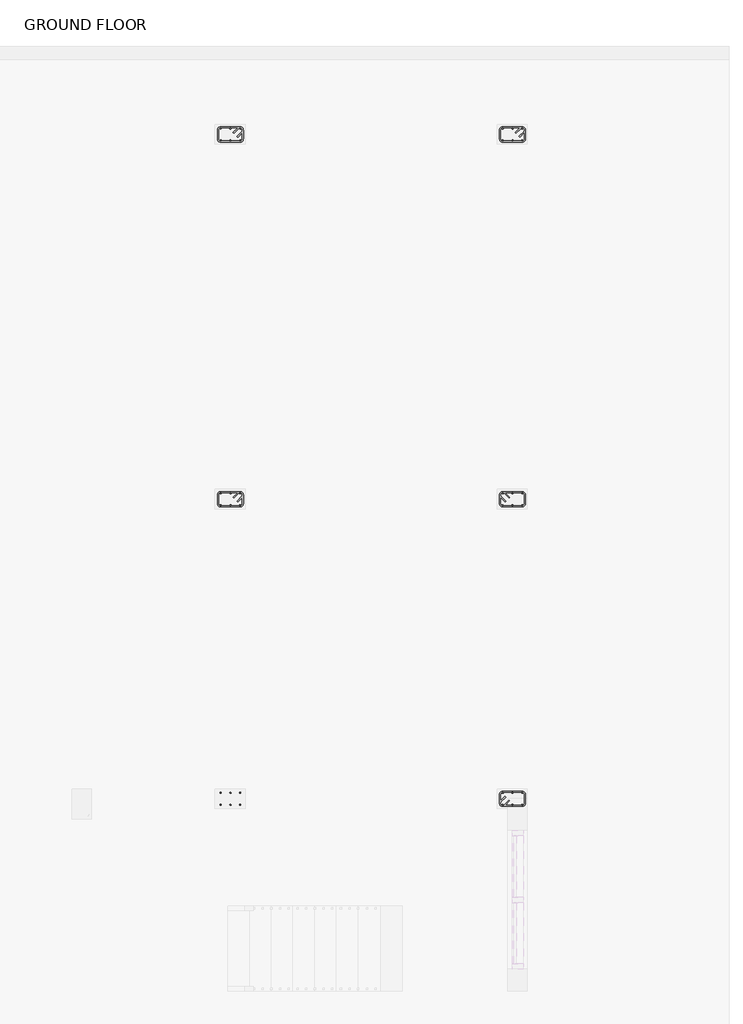
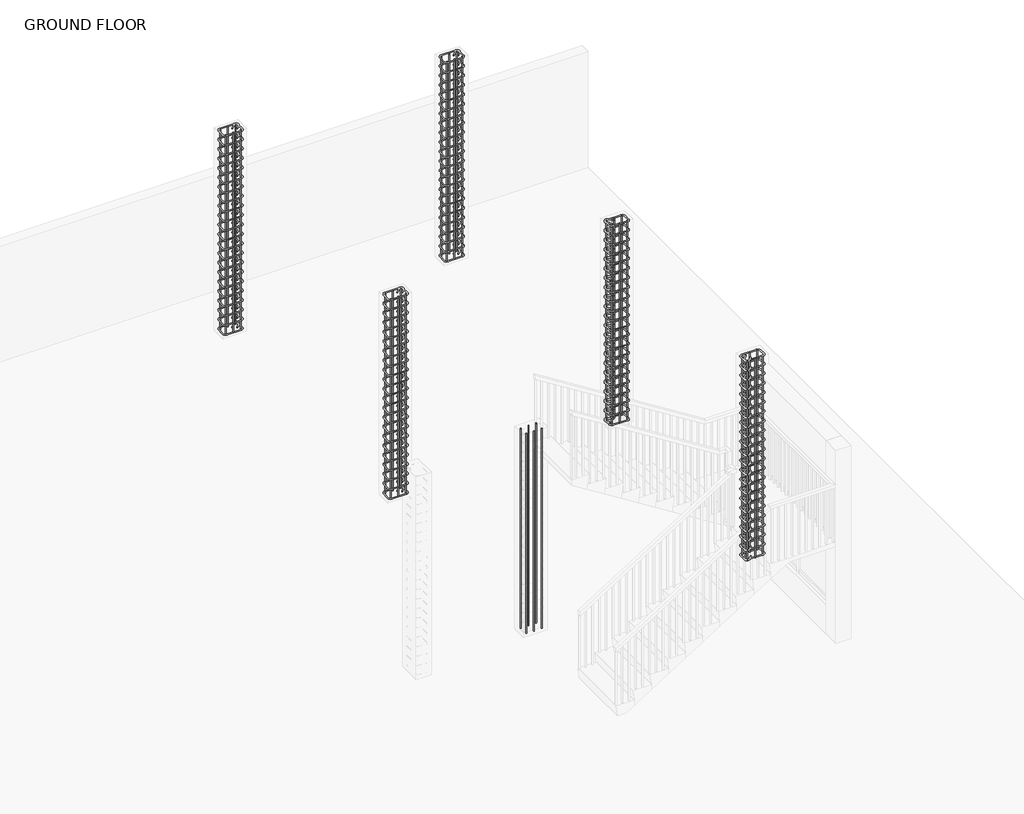
# One storey, part 7 of 7: 17 reinforcing bars.
"""IFC4 building model written with IfcOpenShell, lengths in millimetres."""

from ifc_helpers import new_model, si_unit, point, frame, origin, place, context, project, spatial, polyline, circle_curve, trimmed, segment, composite_curve, source, transform, mapped, element, save
from ifc_brep_helpers import swept_disk

model = new_model("IFC4")

# Units and contexts
model_context = context("Model", 3, world=origin())
ifc_project = project(units=[si_unit("LENGTHUNIT", "METRE", prefix="MILLI")], contexts=[model_context])

# Site, building, storey
site = spatial("IfcSite", under=ifc_project)
building = spatial("IfcBuilding", under=site)
storey = spatial("IfcBuildingStorey", under=building, Name="GROUND FLOOR", Elevation=0.0)

# Reinforcing bars
placement = place(None, origin())
reinforcing_bar_shape = source(origin(), model_context, "Body", "SolidModel", [
    swept_disk(composite_curve([segment(polyline([(4498.0475177, 5737.027757, 3168.65), (4444.165981, 5790.9092937, 3168.65)]), True, "CONTINUOUS"), segment(trimmed(circle_curve(frame((4466.6166213, 5813.359934, 3168.65), z_axis=(0.0, 0.0, -1.0), x_axis=(-22.450640299999577, -22.450640300000487, 0.0)), 31.75), [point((4444.165981, 5790.9092937, 3168.65))], [point((4466.6166213, 5845.109934, 3168.65))], True, "CARTESIAN"), True, "CONTINUOUS"), segment(polyline([(4466.6166213, 5845.109934, 3168.65), (4695.2166213, 5845.109934, 3168.65)]), True, "CONTINUOUS"), segment(trimmed(circle_curve(frame((4695.2166213, 5813.359934, 3168.65), z_axis=(0.0, 0.0, -1.0), x_axis=(0.0, 31.75, 0.0)), 31.75), [point((4695.2166213, 5845.109934, 3168.65))], [point((4726.9666213, 5813.359934, 3168.65))], True, "CARTESIAN"), True, "CONTINUOUS"), segment(polyline([(4726.9666213, 5813.359934, 3168.65), (4726.9666213, 5711.759934, 3168.65)]), True, "CONTINUOUS"), segment(trimmed(circle_curve(frame((4695.2465882, 5711.759934, 3170.0291319), z_axis=(-0.043437224276306856, 0.0, -0.9990561583550596), x_axis=(31.720033100000364, 0.0, -1.3791318999997202)), 31.75), [point((4726.9666213, 5711.759934, 3168.65))], [point((4695.2465882, 5680.009934, 3170.0291319))], True, "CARTESIAN"), True, "CONTINUOUS"), segment(polyline([(4695.2465882, 5680.009934, 3170.0291319), (4466.5866543, 5680.009934, 3179.9708681)]), True, "CONTINUOUS"), segment(trimmed(circle_curve(frame((4466.5866543, 5711.759934, 3179.9708681), z_axis=(-0.043437224276306856, 0.0, -0.9990561583550596), x_axis=(0.0, -31.75, 0.0)), 31.75), [point((4466.5866543, 5680.009934, 3179.9708681))], [point((4434.8666213, 5711.759934, 3181.35))], True, "CARTESIAN"), True, "CONTINUOUS"), segment(polyline([(4434.8666213, 5711.759934, 3181.35), (4434.8666213, 5813.359934, 3181.35)]), True, "CONTINUOUS"), segment(trimmed(circle_curve(frame((4466.6166213, 5813.359934, 3181.35), z_axis=(0.0, 0.0, -1.0), x_axis=(-31.75, 0.0, 0.0)), 31.75), [point((4434.8666213, 5813.359934, 3181.35))], [point((4489.0672616, 5835.8105743, 3181.35))], True, "CARTESIAN"), True, "CONTINUOUS"), segment(polyline([(4489.0672616, 5835.8105743, 3181.35), (4542.9487983, 5781.9290376, 3181.35)]), True, "CONTINUOUS")], self_intersect=False), 6.35),
])
element("IfcReinforcingBar", 1, at=placement, inside=storey, context=model_context, shape_type="MappedRepresentation", body=[
    mapped(reinforcing_bar_shape, transform((0.0, 0.0, 0.0), x_axis=(1.0, 0.0, 0.0), y_axis=(0.0, 1.0, 0.0), z_axis=(0.0, 0.0, 1.0))),
    mapped(reinforcing_bar_shape, transform((0.0, 0.0, -149.3761905), x_axis=(1.0, 0.0, 0.0), y_axis=(0.0, 1.0, 0.0), z_axis=(0.0, 0.0, 1.0))),
    mapped(reinforcing_bar_shape, transform((0.0, 0.0, -298.752381), x_axis=(1.0, 0.0, 0.0), y_axis=(0.0, 1.0, 0.0), z_axis=(0.0, 0.0, 1.0))),
    mapped(reinforcing_bar_shape, transform((0.0, 0.0, -448.1285714), x_axis=(1.0, 0.0, 0.0), y_axis=(0.0, 1.0, 0.0), z_axis=(0.0, 0.0, 1.0))),
    mapped(reinforcing_bar_shape, transform((0.0, 0.0, -597.5047619), x_axis=(1.0, 0.0, 0.0), y_axis=(0.0, 1.0, 0.0), z_axis=(0.0, 0.0, 1.0))),
    mapped(reinforcing_bar_shape, transform((0.0, 0.0, -746.8809524), x_axis=(1.0, 0.0, 0.0), y_axis=(0.0, 1.0, 0.0), z_axis=(0.0, 0.0, 1.0))),
    mapped(reinforcing_bar_shape, transform((0.0, 0.0, -896.2571429), x_axis=(1.0, 0.0, 0.0), y_axis=(0.0, 1.0, 0.0), z_axis=(0.0, 0.0, 1.0))),
    mapped(reinforcing_bar_shape, transform((0.0, 0.0, -1045.6333333), x_axis=(1.0, 0.0, 0.0), y_axis=(0.0, 1.0, 0.0), z_axis=(0.0, 0.0, 1.0))),
    mapped(reinforcing_bar_shape, transform((0.0, 0.0, -1195.0095238), x_axis=(1.0, 0.0, 0.0), y_axis=(0.0, 1.0, 0.0), z_axis=(0.0, 0.0, 1.0))),
    mapped(reinforcing_bar_shape, transform((0.0, 0.0, -1344.3857143), x_axis=(1.0, 0.0, 0.0), y_axis=(0.0, 1.0, 0.0), z_axis=(0.0, 0.0, 1.0))),
    mapped(reinforcing_bar_shape, transform((0.0, 0.0, -1493.7619048), x_axis=(1.0, 0.0, 0.0), y_axis=(0.0, 1.0, 0.0), z_axis=(0.0, 0.0, 1.0))),
    mapped(reinforcing_bar_shape, transform((0.0, 0.0, -1643.1380952), x_axis=(1.0, 0.0, 0.0), y_axis=(0.0, 1.0, 0.0), z_axis=(0.0, 0.0, 1.0))),
    mapped(reinforcing_bar_shape, transform((0.0, 0.0, -1792.5142857), x_axis=(1.0, 0.0, 0.0), y_axis=(0.0, 1.0, 0.0), z_axis=(0.0, 0.0, 1.0))),
    mapped(reinforcing_bar_shape, transform((0.0, 0.0, -1941.8904762), x_axis=(1.0, 0.0, 0.0), y_axis=(0.0, 1.0, 0.0), z_axis=(0.0, 0.0, 1.0))),
    mapped(reinforcing_bar_shape, transform((0.0, 0.0, -2091.2666667), x_axis=(1.0, 0.0, 0.0), y_axis=(0.0, 1.0, 0.0), z_axis=(0.0, 0.0, 1.0))),
    mapped(reinforcing_bar_shape, transform((0.0, 0.0, -2240.6428571), x_axis=(1.0, 0.0, 0.0), y_axis=(0.0, 1.0, 0.0), z_axis=(0.0, 0.0, 1.0))),
    mapped(reinforcing_bar_shape, transform((0.0, 0.0, -2390.0190476), x_axis=(1.0, 0.0, 0.0), y_axis=(0.0, 1.0, 0.0), z_axis=(0.0, 0.0, 1.0))),
    mapped(reinforcing_bar_shape, transform((0.0, 0.0, -2539.3952381), x_axis=(1.0, 0.0, 0.0), y_axis=(0.0, 1.0, 0.0), z_axis=(0.0, 0.0, 1.0))),
    mapped(reinforcing_bar_shape, transform((0.0, 0.0, -2688.7714286), x_axis=(1.0, 0.0, 0.0), y_axis=(0.0, 1.0, 0.0), z_axis=(0.0, 0.0, 1.0))),
    mapped(reinforcing_bar_shape, transform((0.0, 0.0, -2838.147619), x_axis=(1.0, 0.0, 0.0), y_axis=(0.0, 1.0, 0.0), z_axis=(0.0, 0.0, 1.0))),
    mapped(reinforcing_bar_shape, transform((0.0, 0.0, -2987.5238095), x_axis=(1.0, 0.0, 0.0), y_axis=(0.0, 1.0, 0.0), z_axis=(0.0, 0.0, 1.0))),
    mapped(reinforcing_bar_shape, transform((0.0, 0.0, -3136.9), x_axis=(1.0, 0.0, 0.0), y_axis=(0.0, 1.0, 0.0), z_axis=(0.0, 0.0, 1.0))),
])
reinforcing_bar_2_shape = source(origin(), model_context, "Body", "SolidModel", [
    swept_disk(composite_curve([segment(polyline([(4695.2166213, 5692.709934, 3175.0), (4695.2166213, 5692.709934, 25.4)]), True, "CONTINUOUS")], self_intersect=False), 6.35),
])
element("IfcReinforcingBar", 2, at=placement, inside=storey, context=model_context, shape_type="MappedRepresentation", body=[
    mapped(reinforcing_bar_2_shape, transform((0.0, 0.0, 0.0), x_axis=(1.0, 0.0, 0.0), y_axis=(0.0, 1.0, 0.0), z_axis=(0.0, 0.0, 1.0))),
    mapped(reinforcing_bar_2_shape, transform((-114.3, 0.0, 0.0), x_axis=(1.0, 0.0, 0.0), y_axis=(0.0, 1.0, 0.0), z_axis=(0.0, 0.0, 1.0))),
    mapped(reinforcing_bar_2_shape, transform((-228.6, 0.0, 0.0), x_axis=(1.0, 0.0, 0.0), y_axis=(0.0, 1.0, 0.0), z_axis=(0.0, 0.0, 1.0))),
])
reinforcing_bar_3_shape = source(origin(), model_context, "Body", "SolidModel", [
    swept_disk(composite_curve([segment(polyline([(4466.6166213, 5832.409934, 25.4), (4466.6166213, 5832.409934, 3175.0)]), True, "CONTINUOUS")], self_intersect=False), 6.35),
])
element("IfcReinforcingBar", 3, at=placement, inside=storey, context=model_context, shape_type="MappedRepresentation", body=[
    mapped(reinforcing_bar_3_shape, transform((0.0, 0.0, 0.0), x_axis=(1.0, 0.0, 0.0), y_axis=(0.0, 1.0, 0.0), z_axis=(0.0, 0.0, 1.0))),
    mapped(reinforcing_bar_3_shape, transform((114.3, 0.0, 0.0), x_axis=(1.0, 0.0, 0.0), y_axis=(0.0, 1.0, 0.0), z_axis=(0.0, 0.0, 1.0))),
    mapped(reinforcing_bar_3_shape, transform((228.6, 0.0, 0.0), x_axis=(1.0, 0.0, 0.0), y_axis=(0.0, 1.0, 0.0), z_axis=(0.0, 0.0, 1.0))),
])
reinforcing_bar_4_shape = source(origin(), model_context, "Body", "SolidModel", [
    swept_disk(composite_curve([segment(polyline([(1316.8844442, 10049.1290376, 3168.65), (1370.765981, 10103.0105743, 3168.65)]), True, "CONTINUOUS"), segment(trimmed(circle_curve(frame((1393.2166213, 10080.559934, 3168.65), z_axis=(0.0, 0.0, -1.0), x_axis=(-22.450640300000032, 22.450640299999577, 0.0)), 31.75), [point((1370.765981, 10103.0105743, 3168.65))], [point((1424.9666213, 10080.559934, 3168.65))], True, "CARTESIAN"), True, "CONTINUOUS"), segment(polyline([(1424.9666213, 10080.559934, 3168.65), (1424.9666213, 9978.959934, 3168.65)]), True, "CONTINUOUS"), segment(trimmed(circle_curve(frame((1393.2166213, 9978.959934, 3168.65), z_axis=(0.0, 0.0, -1.0), x_axis=(31.75, 0.0, 0.0)), 31.75), [point((1424.9666213, 9978.959934, 3168.65))], [point((1393.2166213, 9947.209934, 3168.65))], True, "CARTESIAN"), True, "CONTINUOUS"), segment(polyline([(1393.2166213, 9947.209934, 3168.65), (1164.6166213, 9947.209934, 3168.65)]), True, "CONTINUOUS"), segment(trimmed(circle_curve(frame((1164.6166213, 9978.8664139, 3171.0851138), z_axis=(0.0, 0.07669649888473773, -0.9970544855015816), x_axis=(0.0, -31.656479899998885, -2.4351137999997263)), 31.75), [point((1164.6166213, 9947.209934, 3168.65))], [point((1132.8666213, 9978.8664139, 3171.0851138))], True, "CARTESIAN"), True, "CONTINUOUS"), segment(polyline([(1132.8666213, 9978.8664139, 3171.0851138), (1132.8666213, 10080.6534541, 3178.9148862)]), True, "CONTINUOUS"), segment(trimmed(circle_curve(frame((1164.6166213, 10080.6534541, 3178.9148862), z_axis=(0.0, 0.07669649888473773, -0.9970544855015816), x_axis=(-31.75, 0.0, 0.0)), 31.75), [point((1132.8666213, 10080.6534541, 3178.9148862))], [point((1164.6166213, 10112.309934, 3181.35))], True, "CARTESIAN"), True, "CONTINUOUS"), segment(polyline([(1164.6166213, 10112.309934, 3181.35), (1393.2166213, 10112.309934, 3181.35)]), True, "CONTINUOUS"), segment(trimmed(circle_curve(frame((1393.2166213, 10080.559934, 3181.35), z_axis=(0.0, 0.0, -1.0), x_axis=(0.0, 31.75, 0.0)), 31.75), [point((1393.2166213, 10112.309934, 3181.35))], [point((1415.6672616, 10058.1092937, 3181.35))], True, "CARTESIAN"), True, "CONTINUOUS"), segment(polyline([(1415.6672616, 10058.1092937, 3181.35), (1361.7857248, 10004.227757, 3181.35)]), True, "CONTINUOUS")], self_intersect=False), 6.35),
])
element("IfcReinforcingBar", 4, at=placement, inside=storey, context=model_context, shape_type="MappedRepresentation", body=[
    mapped(reinforcing_bar_4_shape, transform((0.0, 0.0, 0.0), x_axis=(1.0, 0.0, 0.0), y_axis=(0.0, 1.0, 0.0), z_axis=(0.0, 0.0, 1.0))),
    mapped(reinforcing_bar_4_shape, transform((0.0, 0.0, -149.3761905), x_axis=(1.0, 0.0, 0.0), y_axis=(0.0, 1.0, 0.0), z_axis=(0.0, 0.0, 1.0))),
    mapped(reinforcing_bar_4_shape, transform((0.0, 0.0, -298.752381), x_axis=(1.0, 0.0, 0.0), y_axis=(0.0, 1.0, 0.0), z_axis=(0.0, 0.0, 1.0))),
    mapped(reinforcing_bar_4_shape, transform((0.0, 0.0, -448.1285714), x_axis=(1.0, 0.0, 0.0), y_axis=(0.0, 1.0, 0.0), z_axis=(0.0, 0.0, 1.0))),
    mapped(reinforcing_bar_4_shape, transform((0.0, 0.0, -597.5047619), x_axis=(1.0, 0.0, 0.0), y_axis=(0.0, 1.0, 0.0), z_axis=(0.0, 0.0, 1.0))),
    mapped(reinforcing_bar_4_shape, transform((0.0, 0.0, -746.8809524), x_axis=(1.0, 0.0, 0.0), y_axis=(0.0, 1.0, 0.0), z_axis=(0.0, 0.0, 1.0))),
    mapped(reinforcing_bar_4_shape, transform((0.0, 0.0, -896.2571429), x_axis=(1.0, 0.0, 0.0), y_axis=(0.0, 1.0, 0.0), z_axis=(0.0, 0.0, 1.0))),
    mapped(reinforcing_bar_4_shape, transform((0.0, 0.0, -1045.6333333), x_axis=(1.0, 0.0, 0.0), y_axis=(0.0, 1.0, 0.0), z_axis=(0.0, 0.0, 1.0))),
    mapped(reinforcing_bar_4_shape, transform((0.0, 0.0, -1195.0095238), x_axis=(1.0, 0.0, 0.0), y_axis=(0.0, 1.0, 0.0), z_axis=(0.0, 0.0, 1.0))),
    mapped(reinforcing_bar_4_shape, transform((0.0, 0.0, -1344.3857143), x_axis=(1.0, 0.0, 0.0), y_axis=(0.0, 1.0, 0.0), z_axis=(0.0, 0.0, 1.0))),
    mapped(reinforcing_bar_4_shape, transform((0.0, 0.0, -1493.7619048), x_axis=(1.0, 0.0, 0.0), y_axis=(0.0, 1.0, 0.0), z_axis=(0.0, 0.0, 1.0))),
    mapped(reinforcing_bar_4_shape, transform((0.0, 0.0, -1643.1380952), x_axis=(1.0, 0.0, 0.0), y_axis=(0.0, 1.0, 0.0), z_axis=(0.0, 0.0, 1.0))),
    mapped(reinforcing_bar_4_shape, transform((0.0, 0.0, -1792.5142857), x_axis=(1.0, 0.0, 0.0), y_axis=(0.0, 1.0, 0.0), z_axis=(0.0, 0.0, 1.0))),
    mapped(reinforcing_bar_4_shape, transform((0.0, 0.0, -1941.8904762), x_axis=(1.0, 0.0, 0.0), y_axis=(0.0, 1.0, 0.0), z_axis=(0.0, 0.0, 1.0))),
    mapped(reinforcing_bar_4_shape, transform((0.0, 0.0, -2091.2666667), x_axis=(1.0, 0.0, 0.0), y_axis=(0.0, 1.0, 0.0), z_axis=(0.0, 0.0, 1.0))),
    mapped(reinforcing_bar_4_shape, transform((0.0, 0.0, -2240.6428571), x_axis=(1.0, 0.0, 0.0), y_axis=(0.0, 1.0, 0.0), z_axis=(0.0, 0.0, 1.0))),
    mapped(reinforcing_bar_4_shape, transform((0.0, 0.0, -2390.0190476), x_axis=(1.0, 0.0, 0.0), y_axis=(0.0, 1.0, 0.0), z_axis=(0.0, 0.0, 1.0))),
    mapped(reinforcing_bar_4_shape, transform((0.0, 0.0, -2539.3952381), x_axis=(1.0, 0.0, 0.0), y_axis=(0.0, 1.0, 0.0), z_axis=(0.0, 0.0, 1.0))),
    mapped(reinforcing_bar_4_shape, transform((0.0, 0.0, -2688.7714286), x_axis=(1.0, 0.0, 0.0), y_axis=(0.0, 1.0, 0.0), z_axis=(0.0, 0.0, 1.0))),
    mapped(reinforcing_bar_4_shape, transform((0.0, 0.0, -2838.147619), x_axis=(1.0, 0.0, 0.0), y_axis=(0.0, 1.0, 0.0), z_axis=(0.0, 0.0, 1.0))),
    mapped(reinforcing_bar_4_shape, transform((0.0, 0.0, -2987.5238095), x_axis=(1.0, 0.0, 0.0), y_axis=(0.0, 1.0, 0.0), z_axis=(0.0, 0.0, 1.0))),
    mapped(reinforcing_bar_4_shape, transform((0.0, 0.0, -3136.9), x_axis=(1.0, 0.0, 0.0), y_axis=(0.0, 1.0, 0.0), z_axis=(0.0, 0.0, 1.0))),
])
reinforcing_bar_5_shape = source(origin(), model_context, "Body", "SolidModel", [
    swept_disk(composite_curve([segment(polyline([(1393.2166213, 9959.909934, 3175.0), (1393.2166213, 9959.909934, 25.4)]), True, "CONTINUOUS")], self_intersect=False), 6.35),
])
element("IfcReinforcingBar", 5, at=placement, inside=storey, context=model_context, shape_type="MappedRepresentation", body=[
    mapped(reinforcing_bar_5_shape, transform((0.0, 0.0, 0.0), x_axis=(1.0, 0.0, 0.0), y_axis=(0.0, 1.0, 0.0), z_axis=(0.0, 0.0, 1.0))),
    mapped(reinforcing_bar_5_shape, transform((-114.3, 0.0, 0.0), x_axis=(1.0, 0.0, 0.0), y_axis=(0.0, 1.0, 0.0), z_axis=(0.0, 0.0, 1.0))),
    mapped(reinforcing_bar_5_shape, transform((-228.6, 0.0, 0.0), x_axis=(1.0, 0.0, 0.0), y_axis=(0.0, 1.0, 0.0), z_axis=(0.0, 0.0, 1.0))),
])
reinforcing_bar_6_shape = source(origin(), model_context, "Body", "SolidModel", [
    swept_disk(composite_curve([segment(polyline([(1393.2166213, 10099.609934, 25.4), (1393.2166213, 10099.609934, 3175.0)]), True, "CONTINUOUS")], self_intersect=False), 6.35),
])
element("IfcReinforcingBar", 6, at=placement, inside=storey, context=model_context, shape_type="MappedRepresentation", body=[
    mapped(reinforcing_bar_6_shape, transform((0.0, 0.0, 0.0), x_axis=(1.0, 0.0, 0.0), y_axis=(0.0, 1.0, 0.0), z_axis=(0.0, 0.0, 1.0))),
    mapped(reinforcing_bar_6_shape, transform((-114.3, 0.0, 0.0), x_axis=(1.0, 0.0, 0.0), y_axis=(0.0, 1.0, 0.0), z_axis=(0.0, 0.0, 1.0))),
    mapped(reinforcing_bar_6_shape, transform((-228.6, 0.0, 0.0), x_axis=(1.0, 0.0, 0.0), y_axis=(0.0, 1.0, 0.0), z_axis=(0.0, 0.0, 1.0))),
])
reinforcing_bar_7_shape = source(origin(), model_context, "Body", "SolidModel", [
    swept_disk(composite_curve([segment(polyline([(4618.8844442, 10049.1290376, 3168.65), (4672.765981, 10103.0105743, 3168.65)]), True, "CONTINUOUS"), segment(trimmed(circle_curve(frame((4695.2166213, 10080.559934, 3168.65), z_axis=(0.0, 0.0, -1.0), x_axis=(-22.450640300000487, 22.450640299999577, 0.0)), 31.75), [point((4672.765981, 10103.0105743, 3168.65))], [point((4726.9666213, 10080.559934, 3168.65))], True, "CARTESIAN"), True, "CONTINUOUS"), segment(polyline([(4726.9666213, 10080.559934, 3168.65), (4726.9666213, 9978.959934, 3168.65)]), True, "CONTINUOUS"), segment(trimmed(circle_curve(frame((4695.2166213, 9978.959934, 3168.65), z_axis=(0.0, 0.0, -1.0), x_axis=(31.75, 0.0, 0.0)), 31.75), [point((4726.9666213, 9978.959934, 3168.65))], [point((4695.2166213, 9947.209934, 3168.65))], True, "CARTESIAN"), True, "CONTINUOUS"), segment(polyline([(4695.2166213, 9947.209934, 3168.65), (4466.6166213, 9947.209934, 3168.65)]), True, "CONTINUOUS"), segment(trimmed(circle_curve(frame((4466.6166213, 9978.8664139, 3171.0851138), z_axis=(0.0, 0.07669649888473773, -0.9970544855015816), x_axis=(0.0, -31.656479899998885, -2.4351137999997263)), 31.75), [point((4466.6166213, 9947.209934, 3168.65))], [point((4434.8666213, 9978.8664139, 3171.0851138))], True, "CARTESIAN"), True, "CONTINUOUS"), segment(polyline([(4434.8666213, 9978.8664139, 3171.0851138), (4434.8666213, 10080.6534541, 3178.9148862)]), True, "CONTINUOUS"), segment(trimmed(circle_curve(frame((4466.6166213, 10080.6534541, 3178.9148862), z_axis=(0.0, 0.07669649888473773, -0.9970544855015816), x_axis=(-31.75, 0.0, 0.0)), 31.75), [point((4434.8666213, 10080.6534541, 3178.9148862))], [point((4466.6166213, 10112.309934, 3181.35))], True, "CARTESIAN"), True, "CONTINUOUS"), segment(polyline([(4466.6166213, 10112.309934, 3181.35), (4695.2166213, 10112.309934, 3181.35)]), True, "CONTINUOUS"), segment(trimmed(circle_curve(frame((4695.2166213, 10080.559934, 3181.35), z_axis=(0.0, 0.0, -1.0), x_axis=(0.0, 31.75, 0.0)), 31.75), [point((4695.2166213, 10112.309934, 3181.35))], [point((4717.6672616, 10058.1092937, 3181.35))], True, "CARTESIAN"), True, "CONTINUOUS"), segment(polyline([(4717.6672616, 10058.1092937, 3181.35), (4663.7857248, 10004.227757, 3181.35)]), True, "CONTINUOUS")], self_intersect=False), 6.35),
])
element("IfcReinforcingBar", 7, at=placement, inside=storey, context=model_context, shape_type="MappedRepresentation", body=[
    mapped(reinforcing_bar_7_shape, transform((0.0, 0.0, 0.0), x_axis=(1.0, 0.0, 0.0), y_axis=(0.0, 1.0, 0.0), z_axis=(0.0, 0.0, 1.0))),
    mapped(reinforcing_bar_7_shape, transform((0.0, 0.0, -149.3761905), x_axis=(1.0, 0.0, 0.0), y_axis=(0.0, 1.0, 0.0), z_axis=(0.0, 0.0, 1.0))),
    mapped(reinforcing_bar_7_shape, transform((0.0, 0.0, -298.752381), x_axis=(1.0, 0.0, 0.0), y_axis=(0.0, 1.0, 0.0), z_axis=(0.0, 0.0, 1.0))),
    mapped(reinforcing_bar_7_shape, transform((0.0, 0.0, -448.1285714), x_axis=(1.0, 0.0, 0.0), y_axis=(0.0, 1.0, 0.0), z_axis=(0.0, 0.0, 1.0))),
    mapped(reinforcing_bar_7_shape, transform((0.0, 0.0, -597.5047619), x_axis=(1.0, 0.0, 0.0), y_axis=(0.0, 1.0, 0.0), z_axis=(0.0, 0.0, 1.0))),
    mapped(reinforcing_bar_7_shape, transform((0.0, 0.0, -746.8809524), x_axis=(1.0, 0.0, 0.0), y_axis=(0.0, 1.0, 0.0), z_axis=(0.0, 0.0, 1.0))),
    mapped(reinforcing_bar_7_shape, transform((0.0, 0.0, -896.2571429), x_axis=(1.0, 0.0, 0.0), y_axis=(0.0, 1.0, 0.0), z_axis=(0.0, 0.0, 1.0))),
    mapped(reinforcing_bar_7_shape, transform((0.0, 0.0, -1045.6333333), x_axis=(1.0, 0.0, 0.0), y_axis=(0.0, 1.0, 0.0), z_axis=(0.0, 0.0, 1.0))),
    mapped(reinforcing_bar_7_shape, transform((0.0, 0.0, -1195.0095238), x_axis=(1.0, 0.0, 0.0), y_axis=(0.0, 1.0, 0.0), z_axis=(0.0, 0.0, 1.0))),
    mapped(reinforcing_bar_7_shape, transform((0.0, 0.0, -1344.3857143), x_axis=(1.0, 0.0, 0.0), y_axis=(0.0, 1.0, 0.0), z_axis=(0.0, 0.0, 1.0))),
    mapped(reinforcing_bar_7_shape, transform((0.0, 0.0, -1493.7619048), x_axis=(1.0, 0.0, 0.0), y_axis=(0.0, 1.0, 0.0), z_axis=(0.0, 0.0, 1.0))),
    mapped(reinforcing_bar_7_shape, transform((0.0, 0.0, -1643.1380952), x_axis=(1.0, 0.0, 0.0), y_axis=(0.0, 1.0, 0.0), z_axis=(0.0, 0.0, 1.0))),
    mapped(reinforcing_bar_7_shape, transform((0.0, 0.0, -1792.5142857), x_axis=(1.0, 0.0, 0.0), y_axis=(0.0, 1.0, 0.0), z_axis=(0.0, 0.0, 1.0))),
    mapped(reinforcing_bar_7_shape, transform((0.0, 0.0, -1941.8904762), x_axis=(1.0, 0.0, 0.0), y_axis=(0.0, 1.0, 0.0), z_axis=(0.0, 0.0, 1.0))),
    mapped(reinforcing_bar_7_shape, transform((0.0, 0.0, -2091.2666667), x_axis=(1.0, 0.0, 0.0), y_axis=(0.0, 1.0, 0.0), z_axis=(0.0, 0.0, 1.0))),
    mapped(reinforcing_bar_7_shape, transform((0.0, 0.0, -2240.6428571), x_axis=(1.0, 0.0, 0.0), y_axis=(0.0, 1.0, 0.0), z_axis=(0.0, 0.0, 1.0))),
    mapped(reinforcing_bar_7_shape, transform((0.0, 0.0, -2390.0190476), x_axis=(1.0, 0.0, 0.0), y_axis=(0.0, 1.0, 0.0), z_axis=(0.0, 0.0, 1.0))),
    mapped(reinforcing_bar_7_shape, transform((0.0, 0.0, -2539.3952381), x_axis=(1.0, 0.0, 0.0), y_axis=(0.0, 1.0, 0.0), z_axis=(0.0, 0.0, 1.0))),
    mapped(reinforcing_bar_7_shape, transform((0.0, 0.0, -2688.7714286), x_axis=(1.0, 0.0, 0.0), y_axis=(0.0, 1.0, 0.0), z_axis=(0.0, 0.0, 1.0))),
    mapped(reinforcing_bar_7_shape, transform((0.0, 0.0, -2838.147619), x_axis=(1.0, 0.0, 0.0), y_axis=(0.0, 1.0, 0.0), z_axis=(0.0, 0.0, 1.0))),
    mapped(reinforcing_bar_7_shape, transform((0.0, 0.0, -2987.5238095), x_axis=(1.0, 0.0, 0.0), y_axis=(0.0, 1.0, 0.0), z_axis=(0.0, 0.0, 1.0))),
    mapped(reinforcing_bar_7_shape, transform((0.0, 0.0, -3136.9), x_axis=(1.0, 0.0, 0.0), y_axis=(0.0, 1.0, 0.0), z_axis=(0.0, 0.0, 1.0))),
])
reinforcing_bar_8_shape = source(origin(), model_context, "Body", "SolidModel", [
    swept_disk(composite_curve([segment(polyline([(4695.2166213, 9959.909934, 3175.0), (4695.2166213, 9959.909934, 25.4)]), True, "CONTINUOUS")], self_intersect=False), 6.35),
])
element("IfcReinforcingBar", 8, at=placement, inside=storey, context=model_context, shape_type="MappedRepresentation", body=[
    mapped(reinforcing_bar_8_shape, transform((0.0, 0.0, 0.0), x_axis=(1.0, 0.0, 0.0), y_axis=(0.0, 1.0, 0.0), z_axis=(0.0, 0.0, 1.0))),
    mapped(reinforcing_bar_8_shape, transform((-114.3, 0.0, 0.0), x_axis=(1.0, 0.0, 0.0), y_axis=(0.0, 1.0, 0.0), z_axis=(0.0, 0.0, 1.0))),
    mapped(reinforcing_bar_8_shape, transform((-228.6, 0.0, 0.0), x_axis=(1.0, 0.0, 0.0), y_axis=(0.0, 1.0, 0.0), z_axis=(0.0, 0.0, 1.0))),
])
reinforcing_bar_9_shape = source(origin(), model_context, "Body", "SolidModel", [
    swept_disk(composite_curve([segment(polyline([(4695.2166213, 10099.609934, 25.4), (4695.2166213, 10099.609934, 3175.0)]), True, "CONTINUOUS")], self_intersect=False), 6.35),
])
element("IfcReinforcingBar", 9, at=placement, inside=storey, context=model_context, shape_type="MappedRepresentation", body=[
    mapped(reinforcing_bar_9_shape, transform((0.0, 0.0, 0.0), x_axis=(1.0, 0.0, 0.0), y_axis=(0.0, 1.0, 0.0), z_axis=(0.0, 0.0, 1.0))),
    mapped(reinforcing_bar_9_shape, transform((-114.3, 0.0, 0.0), x_axis=(1.0, 0.0, 0.0), y_axis=(0.0, 1.0, 0.0), z_axis=(0.0, 0.0, 1.0))),
    mapped(reinforcing_bar_9_shape, transform((-228.6, 0.0, 0.0), x_axis=(1.0, 0.0, 0.0), y_axis=(0.0, 1.0, 0.0), z_axis=(0.0, 0.0, 1.0))),
])
reinforcing_bar_10_shape = source(origin(), model_context, "Body", "SolidModel", [
    swept_disk(composite_curve([segment(polyline([(1316.8844442, 5781.9290376, 3168.65), (1370.765981, 5835.8105743, 3168.65)]), True, "CONTINUOUS"), segment(trimmed(circle_curve(frame((1393.2166213, 5813.359934, 3168.65), z_axis=(0.0, 0.0, -1.0), x_axis=(-22.450640300000032, 22.450640299999577, 0.0)), 31.75), [point((1370.765981, 5835.8105743, 3168.65))], [point((1424.9666213, 5813.359934, 3168.65))], True, "CARTESIAN"), True, "CONTINUOUS"), segment(polyline([(1424.9666213, 5813.359934, 3168.65), (1424.9666213, 5711.759934, 3168.65)]), True, "CONTINUOUS"), segment(trimmed(circle_curve(frame((1393.2166213, 5711.759934, 3168.65), z_axis=(0.0, 0.0, -1.0), x_axis=(31.75, 0.0, 0.0)), 31.75), [point((1424.9666213, 5711.759934, 3168.65))], [point((1393.2166213, 5680.009934, 3168.65))], True, "CARTESIAN"), True, "CONTINUOUS"), segment(polyline([(1393.2166213, 5680.009934, 3168.65), (1164.6166213, 5680.009934, 3168.65)]), True, "CONTINUOUS"), segment(trimmed(circle_curve(frame((1164.6166213, 5711.6664139, 3171.0851138), z_axis=(0.0, 0.07669649888473773, -0.9970544855015816), x_axis=(0.0, -31.656479900000704, -2.4351137999997263)), 31.75), [point((1164.6166213, 5680.009934, 3168.65))], [point((1132.8666213, 5711.6664139, 3171.0851138))], True, "CARTESIAN"), True, "CONTINUOUS"), segment(polyline([(1132.8666213, 5711.6664139, 3171.0851138), (1132.8666213, 5813.4534541, 3178.9148862)]), True, "CONTINUOUS"), segment(trimmed(circle_curve(frame((1164.6166213, 5813.4534541, 3178.9148862), z_axis=(0.0, 0.07669649888473773, -0.9970544855015816), x_axis=(-31.75, 0.0, 0.0)), 31.75), [point((1132.8666213, 5813.4534541, 3178.9148862))], [point((1164.6166213, 5845.109934, 3181.35))], True, "CARTESIAN"), True, "CONTINUOUS"), segment(polyline([(1164.6166213, 5845.109934, 3181.35), (1393.2166213, 5845.109934, 3181.35)]), True, "CONTINUOUS"), segment(trimmed(circle_curve(frame((1393.2166213, 5813.359934, 3181.35), z_axis=(0.0, 0.0, -1.0), x_axis=(0.0, 31.75, 0.0)), 31.75), [point((1393.2166213, 5845.109934, 3181.35))], [point((1415.6672616, 5790.9092937, 3181.35))], True, "CARTESIAN"), True, "CONTINUOUS"), segment(polyline([(1415.6672616, 5790.9092937, 3181.35), (1361.7857248, 5737.027757, 3181.35)]), True, "CONTINUOUS")], self_intersect=False), 6.35),
])
element("IfcReinforcingBar", 10, at=placement, inside=storey, context=model_context, shape_type="MappedRepresentation", body=[
    mapped(reinforcing_bar_10_shape, transform((0.0, 0.0, 0.0), x_axis=(1.0, 0.0, 0.0), y_axis=(0.0, 1.0, 0.0), z_axis=(0.0, 0.0, 1.0))),
    mapped(reinforcing_bar_10_shape, transform((0.0, 0.0, -149.3761905), x_axis=(1.0, 0.0, 0.0), y_axis=(0.0, 1.0, 0.0), z_axis=(0.0, 0.0, 1.0))),
    mapped(reinforcing_bar_10_shape, transform((0.0, 0.0, -298.752381), x_axis=(1.0, 0.0, 0.0), y_axis=(0.0, 1.0, 0.0), z_axis=(0.0, 0.0, 1.0))),
    mapped(reinforcing_bar_10_shape, transform((0.0, 0.0, -448.1285714), x_axis=(1.0, 0.0, 0.0), y_axis=(0.0, 1.0, 0.0), z_axis=(0.0, 0.0, 1.0))),
    mapped(reinforcing_bar_10_shape, transform((0.0, 0.0, -597.5047619), x_axis=(1.0, 0.0, 0.0), y_axis=(0.0, 1.0, 0.0), z_axis=(0.0, 0.0, 1.0))),
    mapped(reinforcing_bar_10_shape, transform((0.0, 0.0, -746.8809524), x_axis=(1.0, 0.0, 0.0), y_axis=(0.0, 1.0, 0.0), z_axis=(0.0, 0.0, 1.0))),
    mapped(reinforcing_bar_10_shape, transform((0.0, 0.0, -896.2571429), x_axis=(1.0, 0.0, 0.0), y_axis=(0.0, 1.0, 0.0), z_axis=(0.0, 0.0, 1.0))),
    mapped(reinforcing_bar_10_shape, transform((0.0, 0.0, -1045.6333333), x_axis=(1.0, 0.0, 0.0), y_axis=(0.0, 1.0, 0.0), z_axis=(0.0, 0.0, 1.0))),
    mapped(reinforcing_bar_10_shape, transform((0.0, 0.0, -1195.0095238), x_axis=(1.0, 0.0, 0.0), y_axis=(0.0, 1.0, 0.0), z_axis=(0.0, 0.0, 1.0))),
    mapped(reinforcing_bar_10_shape, transform((0.0, 0.0, -1344.3857143), x_axis=(1.0, 0.0, 0.0), y_axis=(0.0, 1.0, 0.0), z_axis=(0.0, 0.0, 1.0))),
    mapped(reinforcing_bar_10_shape, transform((0.0, 0.0, -1493.7619048), x_axis=(1.0, 0.0, 0.0), y_axis=(0.0, 1.0, 0.0), z_axis=(0.0, 0.0, 1.0))),
    mapped(reinforcing_bar_10_shape, transform((0.0, 0.0, -1643.1380952), x_axis=(1.0, 0.0, 0.0), y_axis=(0.0, 1.0, 0.0), z_axis=(0.0, 0.0, 1.0))),
    mapped(reinforcing_bar_10_shape, transform((0.0, 0.0, -1792.5142857), x_axis=(1.0, 0.0, 0.0), y_axis=(0.0, 1.0, 0.0), z_axis=(0.0, 0.0, 1.0))),
    mapped(reinforcing_bar_10_shape, transform((0.0, 0.0, -1941.8904762), x_axis=(1.0, 0.0, 0.0), y_axis=(0.0, 1.0, 0.0), z_axis=(0.0, 0.0, 1.0))),
    mapped(reinforcing_bar_10_shape, transform((0.0, 0.0, -2091.2666667), x_axis=(1.0, 0.0, 0.0), y_axis=(0.0, 1.0, 0.0), z_axis=(0.0, 0.0, 1.0))),
    mapped(reinforcing_bar_10_shape, transform((0.0, 0.0, -2240.6428571), x_axis=(1.0, 0.0, 0.0), y_axis=(0.0, 1.0, 0.0), z_axis=(0.0, 0.0, 1.0))),
    mapped(reinforcing_bar_10_shape, transform((0.0, 0.0, -2390.0190476), x_axis=(1.0, 0.0, 0.0), y_axis=(0.0, 1.0, 0.0), z_axis=(0.0, 0.0, 1.0))),
    mapped(reinforcing_bar_10_shape, transform((0.0, 0.0, -2539.3952381), x_axis=(1.0, 0.0, 0.0), y_axis=(0.0, 1.0, 0.0), z_axis=(0.0, 0.0, 1.0))),
    mapped(reinforcing_bar_10_shape, transform((0.0, 0.0, -2688.7714286), x_axis=(1.0, 0.0, 0.0), y_axis=(0.0, 1.0, 0.0), z_axis=(0.0, 0.0, 1.0))),
    mapped(reinforcing_bar_10_shape, transform((0.0, 0.0, -2838.147619), x_axis=(1.0, 0.0, 0.0), y_axis=(0.0, 1.0, 0.0), z_axis=(0.0, 0.0, 1.0))),
    mapped(reinforcing_bar_10_shape, transform((0.0, 0.0, -2987.5238095), x_axis=(1.0, 0.0, 0.0), y_axis=(0.0, 1.0, 0.0), z_axis=(0.0, 0.0, 1.0))),
    mapped(reinforcing_bar_10_shape, transform((0.0, 0.0, -3136.9), x_axis=(1.0, 0.0, 0.0), y_axis=(0.0, 1.0, 0.0), z_axis=(0.0, 0.0, 1.0))),
])
reinforcing_bar_11_shape = source(origin(), model_context, "Body", "SolidModel", [
    swept_disk(composite_curve([segment(polyline([(1393.2166213, 5692.709934, 3175.0), (1393.2166213, 5692.709934, 25.4)]), True, "CONTINUOUS")], self_intersect=False), 6.35),
])
element("IfcReinforcingBar", 11, at=placement, inside=storey, context=model_context, shape_type="MappedRepresentation", body=[
    mapped(reinforcing_bar_11_shape, transform((0.0, 0.0, 0.0), x_axis=(1.0, 0.0, 0.0), y_axis=(0.0, 1.0, 0.0), z_axis=(0.0, 0.0, 1.0))),
    mapped(reinforcing_bar_11_shape, transform((-114.3, 0.0, 0.0), x_axis=(1.0, 0.0, 0.0), y_axis=(0.0, 1.0, 0.0), z_axis=(0.0, 0.0, 1.0))),
    mapped(reinforcing_bar_11_shape, transform((-228.6, 0.0, 0.0), x_axis=(1.0, 0.0, 0.0), y_axis=(0.0, 1.0, 0.0), z_axis=(0.0, 0.0, 1.0))),
])
reinforcing_bar_12_shape = source(origin(), model_context, "Body", "SolidModel", [
    swept_disk(composite_curve([segment(polyline([(1393.2166213, 5832.409934, 25.4), (1393.2166213, 5832.409934, 3175.0)]), True, "CONTINUOUS")], self_intersect=False), 6.35),
])
element("IfcReinforcingBar", 12, at=placement, inside=storey, context=model_context, shape_type="MappedRepresentation", body=[
    mapped(reinforcing_bar_12_shape, transform((0.0, 0.0, 0.0), x_axis=(1.0, 0.0, 0.0), y_axis=(0.0, 1.0, 0.0), z_axis=(0.0, 0.0, 1.0))),
    mapped(reinforcing_bar_12_shape, transform((-114.3, 0.0, 0.0), x_axis=(1.0, 0.0, 0.0), y_axis=(0.0, 1.0, 0.0), z_axis=(0.0, 0.0, 1.0))),
    mapped(reinforcing_bar_12_shape, transform((-228.6, 0.0, 0.0), x_axis=(1.0, 0.0, 0.0), y_axis=(0.0, 1.0, 0.0), z_axis=(0.0, 0.0, 1.0))),
])
reinforcing_bar_13_shape = source(origin(), model_context, "Body", "SolidModel", [
    swept_disk(composite_curve([segment(polyline([(1164.6166213, 2327.209934, 3175.0), (1164.6166213, 2327.209934, 25.4)]), True, "CONTINUOUS")], self_intersect=False), 6.35),
])
element("IfcReinforcingBar", 13, at=placement, inside=storey, context=model_context, shape_type="MappedRepresentation", body=[
    mapped(reinforcing_bar_13_shape, transform((0.0, 0.0, 0.0), x_axis=(1.0, 0.0, 0.0), y_axis=(0.0, 1.0, 0.0), z_axis=(0.0, 0.0, 1.0))),
    mapped(reinforcing_bar_13_shape, transform((114.3, 0.0, 0.0), x_axis=(1.0, 0.0, 0.0), y_axis=(0.0, 1.0, 0.0), z_axis=(0.0, 0.0, 1.0))),
    mapped(reinforcing_bar_13_shape, transform((228.6, 0.0, 0.0), x_axis=(1.0, 0.0, 0.0), y_axis=(0.0, 1.0, 0.0), z_axis=(0.0, 0.0, 1.0))),
])
reinforcing_bar_14_shape = source(origin(), model_context, "Body", "SolidModel", [
    swept_disk(composite_curve([segment(polyline([(1164.6166213, 2187.509934, 25.4), (1164.6166213, 2187.509934, 3175.0)]), True, "CONTINUOUS")], self_intersect=False), 6.35),
])
element("IfcReinforcingBar", 14, at=placement, inside=storey, context=model_context, shape_type="MappedRepresentation", body=[
    mapped(reinforcing_bar_14_shape, transform((0.0, 0.0, 0.0), x_axis=(1.0, 0.0, 0.0), y_axis=(0.0, 1.0, 0.0), z_axis=(0.0, 0.0, 1.0))),
    mapped(reinforcing_bar_14_shape, transform((114.3, 0.0, 0.0), x_axis=(1.0, 0.0, 0.0), y_axis=(0.0, 1.0, 0.0), z_axis=(0.0, 0.0, 1.0))),
    mapped(reinforcing_bar_14_shape, transform((228.6, 0.0, 0.0), x_axis=(1.0, 0.0, 0.0), y_axis=(0.0, 1.0, 0.0), z_axis=(0.0, 0.0, 1.0))),
])
reinforcing_bar_15_shape = source(origin(), model_context, "Body", "SolidModel", [
    swept_disk(composite_curve([segment(polyline([(4542.9487983, 2237.9908305, 3168.65), (4489.0672616, 2184.1092937, 3168.65)]), True, "CONTINUOUS"), segment(trimmed(circle_curve(frame((4466.6166213, 2206.559934, 3168.65), z_axis=(0.0, 0.0, -1.0), x_axis=(22.450640300000487, -22.450640300000032, 0.0)), 31.75), [point((4489.0672616, 2184.1092937, 3168.65))], [point((4434.8666213, 2206.559934, 3168.65))], True, "CARTESIAN"), True, "CONTINUOUS"), segment(polyline([(4434.8666213, 2206.559934, 3168.65), (4434.8666213, 2308.159934, 3168.65)]), True, "CONTINUOUS"), segment(trimmed(circle_curve(frame((4466.6166213, 2308.159934, 3168.65), z_axis=(0.0, 0.0, -1.0), x_axis=(-31.75, 0.0, 0.0)), 31.75), [point((4434.8666213, 2308.159934, 3168.65))], [point((4466.6166213, 2339.909934, 3168.65))], True, "CARTESIAN"), True, "CONTINUOUS"), segment(polyline([(4466.6166213, 2339.909934, 3168.65), (4695.2166213, 2339.909934, 3168.65)]), True, "CONTINUOUS"), segment(trimmed(circle_curve(frame((4695.2166213, 2308.2534541, 3171.0851138), z_axis=(0.0, -0.07669649888473773, -0.9970544855015816), x_axis=(0.0, 31.656479899999795, -2.4351137999997263)), 31.75), [point((4695.2166213, 2339.909934, 3168.65))], [point((4726.9666213, 2308.2534541, 3171.0851138))], True, "CARTESIAN"), True, "CONTINUOUS"), segment(polyline([(4726.9666213, 2308.2534541, 3171.0851138), (4726.9666213, 2206.4664139, 3178.9148862)]), True, "CONTINUOUS"), segment(trimmed(circle_curve(frame((4695.2166213, 2206.4664139, 3178.9148862), z_axis=(0.0, -0.07669649888473773, -0.9970544855015816), x_axis=(31.75, 0.0, 0.0)), 31.75), [point((4726.9666213, 2206.4664139, 3178.9148862))], [point((4695.2166213, 2174.809934, 3181.35))], True, "CARTESIAN"), True, "CONTINUOUS"), segment(polyline([(4695.2166213, 2174.809934, 3181.35), (4466.6166213, 2174.809934, 3181.35)]), True, "CONTINUOUS"), segment(trimmed(circle_curve(frame((4466.6166213, 2206.559934, 3181.35), z_axis=(0.0, 0.0, -1.0), x_axis=(0.0, -31.75, 0.0)), 31.75), [point((4466.6166213, 2174.809934, 3181.35))], [point((4444.165981, 2229.0105743, 3181.35))], True, "CARTESIAN"), True, "CONTINUOUS"), segment(polyline([(4444.165981, 2229.0105743, 3181.35), (4498.0475177, 2282.8921111, 3181.35)]), True, "CONTINUOUS")], self_intersect=False), 6.35),
])
element("IfcReinforcingBar", 15, at=placement, inside=storey, context=model_context, shape_type="MappedRepresentation", body=[
    mapped(reinforcing_bar_15_shape, transform((0.0, 0.0, 0.0), x_axis=(1.0, 0.0, 0.0), y_axis=(0.0, 1.0, 0.0), z_axis=(0.0, 0.0, 1.0))),
    mapped(reinforcing_bar_15_shape, transform((0.0, 0.0, -149.3761905), x_axis=(1.0, 0.0, 0.0), y_axis=(0.0, 1.0, 0.0), z_axis=(0.0, 0.0, 1.0))),
    mapped(reinforcing_bar_15_shape, transform((0.0, 0.0, -298.752381), x_axis=(1.0, 0.0, 0.0), y_axis=(0.0, 1.0, 0.0), z_axis=(0.0, 0.0, 1.0))),
    mapped(reinforcing_bar_15_shape, transform((0.0, 0.0, -448.1285714), x_axis=(1.0, 0.0, 0.0), y_axis=(0.0, 1.0, 0.0), z_axis=(0.0, 0.0, 1.0))),
    mapped(reinforcing_bar_15_shape, transform((0.0, 0.0, -597.5047619), x_axis=(1.0, 0.0, 0.0), y_axis=(0.0, 1.0, 0.0), z_axis=(0.0, 0.0, 1.0))),
    mapped(reinforcing_bar_15_shape, transform((0.0, 0.0, -746.8809524), x_axis=(1.0, 0.0, 0.0), y_axis=(0.0, 1.0, 0.0), z_axis=(0.0, 0.0, 1.0))),
    mapped(reinforcing_bar_15_shape, transform((0.0, 0.0, -896.2571429), x_axis=(1.0, 0.0, 0.0), y_axis=(0.0, 1.0, 0.0), z_axis=(0.0, 0.0, 1.0))),
    mapped(reinforcing_bar_15_shape, transform((0.0, 0.0, -1045.6333333), x_axis=(1.0, 0.0, 0.0), y_axis=(0.0, 1.0, 0.0), z_axis=(0.0, 0.0, 1.0))),
    mapped(reinforcing_bar_15_shape, transform((0.0, 0.0, -1195.0095238), x_axis=(1.0, 0.0, 0.0), y_axis=(0.0, 1.0, 0.0), z_axis=(0.0, 0.0, 1.0))),
    mapped(reinforcing_bar_15_shape, transform((0.0, 0.0, -1344.3857143), x_axis=(1.0, 0.0, 0.0), y_axis=(0.0, 1.0, 0.0), z_axis=(0.0, 0.0, 1.0))),
    mapped(reinforcing_bar_15_shape, transform((0.0, 0.0, -1493.7619048), x_axis=(1.0, 0.0, 0.0), y_axis=(0.0, 1.0, 0.0), z_axis=(0.0, 0.0, 1.0))),
    mapped(reinforcing_bar_15_shape, transform((0.0, 0.0, -1643.1380952), x_axis=(1.0, 0.0, 0.0), y_axis=(0.0, 1.0, 0.0), z_axis=(0.0, 0.0, 1.0))),
    mapped(reinforcing_bar_15_shape, transform((0.0, 0.0, -1792.5142857), x_axis=(1.0, 0.0, 0.0), y_axis=(0.0, 1.0, 0.0), z_axis=(0.0, 0.0, 1.0))),
    mapped(reinforcing_bar_15_shape, transform((0.0, 0.0, -1941.8904762), x_axis=(1.0, 0.0, 0.0), y_axis=(0.0, 1.0, 0.0), z_axis=(0.0, 0.0, 1.0))),
    mapped(reinforcing_bar_15_shape, transform((0.0, 0.0, -2091.2666667), x_axis=(1.0, 0.0, 0.0), y_axis=(0.0, 1.0, 0.0), z_axis=(0.0, 0.0, 1.0))),
    mapped(reinforcing_bar_15_shape, transform((0.0, 0.0, -2240.6428571), x_axis=(1.0, 0.0, 0.0), y_axis=(0.0, 1.0, 0.0), z_axis=(0.0, 0.0, 1.0))),
    mapped(reinforcing_bar_15_shape, transform((0.0, 0.0, -2390.0190476), x_axis=(1.0, 0.0, 0.0), y_axis=(0.0, 1.0, 0.0), z_axis=(0.0, 0.0, 1.0))),
    mapped(reinforcing_bar_15_shape, transform((0.0, 0.0, -2539.3952381), x_axis=(1.0, 0.0, 0.0), y_axis=(0.0, 1.0, 0.0), z_axis=(0.0, 0.0, 1.0))),
    mapped(reinforcing_bar_15_shape, transform((0.0, 0.0, -2688.7714286), x_axis=(1.0, 0.0, 0.0), y_axis=(0.0, 1.0, 0.0), z_axis=(0.0, 0.0, 1.0))),
    mapped(reinforcing_bar_15_shape, transform((0.0, 0.0, -2838.147619), x_axis=(1.0, 0.0, 0.0), y_axis=(0.0, 1.0, 0.0), z_axis=(0.0, 0.0, 1.0))),
    mapped(reinforcing_bar_15_shape, transform((0.0, 0.0, -2987.5238095), x_axis=(1.0, 0.0, 0.0), y_axis=(0.0, 1.0, 0.0), z_axis=(0.0, 0.0, 1.0))),
    mapped(reinforcing_bar_15_shape, transform((0.0, 0.0, -3136.9), x_axis=(1.0, 0.0, 0.0), y_axis=(0.0, 1.0, 0.0), z_axis=(0.0, 0.0, 1.0))),
])
reinforcing_bar_16_shape = source(origin(), model_context, "Body", "SolidModel", [
    swept_disk(composite_curve([segment(polyline([(4466.6166213, 2327.209934, 3175.0), (4466.6166213, 2327.209934, 25.4)]), True, "CONTINUOUS")], self_intersect=False), 6.35),
])
element("IfcReinforcingBar", 16, at=placement, inside=storey, context=model_context, shape_type="MappedRepresentation", body=[
    mapped(reinforcing_bar_16_shape, transform((0.0, 0.0, 0.0), x_axis=(1.0, 0.0, 0.0), y_axis=(0.0, 1.0, 0.0), z_axis=(0.0, 0.0, 1.0))),
    mapped(reinforcing_bar_16_shape, transform((114.3, 0.0, 0.0), x_axis=(1.0, 0.0, 0.0), y_axis=(0.0, 1.0, 0.0), z_axis=(0.0, 0.0, 1.0))),
    mapped(reinforcing_bar_16_shape, transform((228.6, 0.0, 0.0), x_axis=(1.0, 0.0, 0.0), y_axis=(0.0, 1.0, 0.0), z_axis=(0.0, 0.0, 1.0))),
])
reinforcing_bar_17_shape = source(origin(), model_context, "Body", "SolidModel", [
    swept_disk(composite_curve([segment(polyline([(4466.6166213, 2187.509934, 25.4), (4466.6166213, 2187.509934, 3175.0)]), True, "CONTINUOUS")], self_intersect=False), 6.35),
])
element("IfcReinforcingBar", 17, at=placement, inside=storey, context=model_context, shape_type="MappedRepresentation", body=[
    mapped(reinforcing_bar_17_shape, transform((0.0, 0.0, 0.0), x_axis=(1.0, 0.0, 0.0), y_axis=(0.0, 1.0, 0.0), z_axis=(0.0, 0.0, 1.0))),
    mapped(reinforcing_bar_17_shape, transform((114.3, 0.0, 0.0), x_axis=(1.0, 0.0, 0.0), y_axis=(0.0, 1.0, 0.0), z_axis=(0.0, 0.0, 1.0))),
    mapped(reinforcing_bar_17_shape, transform((228.6, 0.0, 0.0), x_axis=(1.0, 0.0, 0.0), y_axis=(0.0, 1.0, 0.0), z_axis=(0.0, 0.0, 1.0))),
])

save(model, "model.ifc")

# Revit data of these elements
# Elements 1, 2, 3, 4, 5, 6, 7, 8, 9, 10, 11, 12, 13, 14, 15, 16, 17 (IfcReinforcingBar)
#   Phase Created = New Construction
